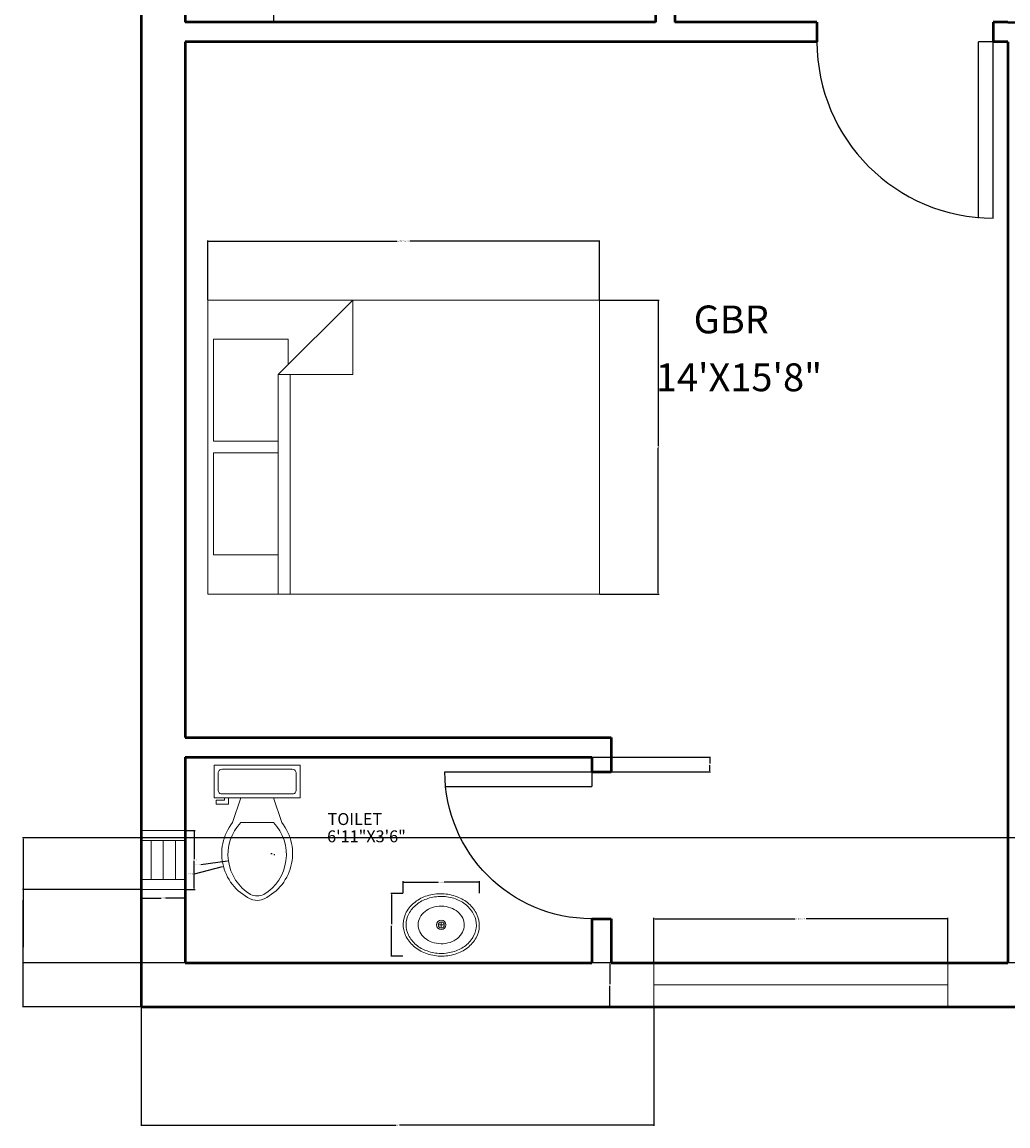
# Model space of a CAD drawing. Units: inches. Extents: x 66 to 499, y 601 to 1111.
# Tile 1 of 4: x 66 to 268, y 601 to 826. Entities that reach past the tile are written whole.
import ezdxf

# ---------------------------------------------------------------- set-up
doc = ezdxf.new("R2010")
doc.units = ezdxf.units.IN
for name, color, linetype, lineweight in [('A-ANNO-DIMS', 2, 'Continuous', 18), ('A-AREA-IDEN', 7, 'Continuous', 18), ('A-DOOR', 3, 'Continuous', 25), ('A-FLOR-CASE', 9, 'Continuous', 25), ('A-FLOR-FIXT', 9, 'Continuous', 18), ('A-FURN', 8, 'Continuous', 18), ('A-GLAZ', 4, 'Continuous', 18), ('A-WALL', 7, 'Continuous', 50)]:
    doc.layers.add(name, color=color, linetype=linetype, lineweight=lineweight)
doc.styles.get("Standard").update_dxf_attribs({"font": 'arial.ttf'})
doc.dimstyles.get("Standard").update_dxf_attribs({"dimtxt": 0.18, "dimasz": 0.18, "dimexe": 0.18, "dimexo": 0.0625, "dimgap": 0.09, "dimtad": 0, "dimtih": 1, "dimtoh": 1, "dimdec": 4, "dimzin": 0, "dimdsep": 46, "dimtxsty": 'Standard', "dimcen": 0.09, "dimadec": 0, "dimazin": 0, "dimtfac": 1, "dimtdec": 4, "dimtofl": 0, "dimtmove": 0, "dimatfit": 3, "dimfxl": 1, "dimtolj": 1, "dimtzin": 0, "dimarcsym": 0})

# ---------------------------------------------------------------- blocks, each defined once
blk = doc.blocks.new('Toilet - top')
for p, q in [((9.5, -6), (9.5, -2)), ((-8, -8.5), (-8, -8)), ((-7, -8), (-7, -9.5)), ((-4, -8), (-6, -14)), ((4, -8), (6, -14)), ((-10, -8.5), (-8, -8.5)), ((-10, -9.5), (-10, -8.5)), ((-7, -9.5), (-10, -9.5)), ((4, -14), (-4, -14))]:
    blk.add_line(p, q)
blk.add_lwpolyline([(10.5, -8), (10.5, 0), (-10.5, 0), (-10.5, -8)], close=True)
for points in [[(-9.5, -2), (-9.5, -6)], [(8.5, -1), (-8.5, -1)], [(-8.5, -7), (8.5, -7)]]:
    blk.add_lwpolyline(points)
for centre, radius, start, end in [((-8.62, -1.88), 0.884, 81.8699, 188.1301), ((8.62, -1.88), 0.884, 351.8699, 98.1301), ((-8.62, -6.12), 0.884, 171.8699, 278.1301), ((8.62, -6.12), 0.884, 261.8699, 8.1301), ((3.52, -21.58), 12.17, 141.4691, 247.9714), ((4.2, -21.82), 11.33, 136.3677, 238.9468), ((-3.52, -21.58), 12.17, 292.0284, 38.5307), ((-4.2, -21.82), 11.33, 301.053, 43.6321), ((0, -27.88), 4, 245.7318, 294.2682), ((0, -29), 4, 254.8605, 285.1395)]:
    blk.add_arc(centre, radius, start, end)
blk = doc.blocks.new('Sink - Oval top')
for p, q in [((-1, 0), (1, 0)), ((0, 1), (0, -1))]:
    blk.add_line(p, q)
for points in [[(-12.23, 0.39, 0.117634), (-11.46, -3.36, 0.104469), (-8.88, -6.8, 0.090016), (-5.08, -9.07, 0.08192), (-0.32, -10.02, 0.08192), (4.49, -9.38, 0.090016), (8.42, -7.36, 0.104469), (11.22, -4.09, 0.117634), (12.23, -0.39, 0.117634), (11.46, 3.36, 0.104469), (8.88, 6.8, 0.090016), (5.08, 9.07, 0.08192), (0.32, 10.02, 0.08192), (-4.49, 9.38, 0.090016), (-8.42, 7.36, 0.104469), (-11.22, 4.09, 0.117634)], [(-11.29, 0.16, 0.118622), (-10.52, -3.25, 0.104678), (-8.07, -6.36, 0.089562), (-4.54, -8.37, 0.081185), (-0.13, -9.15, 0.081185), (4.3, -8.49, 0.089562), (7.89, -6.58, 0.104678), (10.42, -3.55, 0.118622), (11.29, -0.16, 0.118622), (10.52, 3.25, 0.104678), (8.07, 6.36, 0.089562), (4.54, 8.37, 0.081185), (0.13, 9.15, 0.081185), (-4.3, 8.49, 0.089562), (-7.89, 6.58, 0.104678), (-10.42, 3.55, 0.118622)], [(-7.42, 0.08, 0.118283), (-6.91, -2.17, 0.104607), (-5.29, -4.21, 0.089718), (-2.97, -5.53, 0.081436), (-0.07, -6.04, 0.081436), (2.84, -5.59, 0.089718), (5.2, -4.33, 0.104607), (6.86, -2.32, 0.118283), (7.42, -0.08, 0.118283), (6.91, 2.17, 0.104607), (5.29, 4.21, 0.089718), (2.97, 5.53, 0.081436), (0.07, 6.04, 0.081436), (-2.84, 5.59, 0.089718), (-5.2, 4.33, 0.104607), (-6.86, 2.32, 0.118283)]]:
    blk.add_lwpolyline(points, format="xyb", close=True)
for radius in [1.5, 1]:
    blk.add_circle((0, 0), radius)
blk = doc.blocks.new('Bed - Queen')
for p, q in [((0, -80.00003), (0, 0)), ((0, 0), (59.99999, 0)), ((59.99999, 0), (59.99999, -80.00003)), ((7.99999, -1.2), (28.79998, -1.2)), ((7.99999, -14.4), (7.99999, -1.2)), ((28.79998, -1.2), (28.79998, -14.4)), ((31.19999, -1.2), (51.99999, -1.2)), ((31.19999, -14.4), (31.19999, -1.2)), ((51.99999, -1.2), (51.99999, -16.4)), ((0, -14.4), (44.8, -14.4)), ((59.99999, -29.6), (44.8, -14.4)), ((44.8, -14.4), (44.8, -29.6)), ((44.8, -16.8), (0, -16.8)), ((51.99999, -16.4), (46.79936, -16.4)), ((44.8, -29.6), (59.99999, -29.6)), ((59.99999, -80.00003), (0, -80.00003))]:
    blk.add_line(p, q)
blk = doc.blocks.new('DOOR-SWING-36IN')
for p, q in [((0, 36), (0, 0)), ((3, 36), (3, 0)), ((0, 0), (3, 0))]:
    blk.add_line(p, q)
blk.add_arc((0, 0), 36, 0, 90)
blk = doc.blocks.new('DOOR-SWING-30IN')
for p, q in [((0, 30), (0, 0)), ((3, 30), (3, 0)), ((0, 0), (3, 0.01))]:
    blk.add_line(p, q)
blk.add_arc((0, 0), 30, 0.0977, 90)
blk = doc.blocks.new('WIN-60IN')
for p, q in [((60, 9), (0, 9)), ((0, 9), (0, 0)), ((60, 0), (60, 9)), ((0, 4.5), (60, 4.5)), ((0, 0), (60, 0))]:
    blk.add_line(p, q)
blk = doc.blocks.new('WIN-BATH-VENT-12IN')
for p, q in [((0, 12), (0, 0)), ((9, 12), (0, 12)), ((9, 0), (9, 12)), ((9, 10), (0, 10)), ((2, 10), (2, 2)), ((4.5, 10), (4.5, 2)), ((7, 2), (7, 10)), ((0, 2), (9, 2)), ((0, 0), (9, 0))]:
    blk.add_line(p, q)
blk = doc.blocks.new('*D14')
at = {"layer": 'A-ANNO-DIMS', "color": 0, "lineweight": -2, "transparency": 16777216}
for p, q in [((195.27, 634.07), (195.27, 643.18)), ((195.45, 643), (224.15, 643)), ((255.09, 643), (226.39, 643)), ((255.27, 634.07), (255.27, 643.18))]:
    blk.add_line(p, q, dxfattribs=at)
at = {"layer": 'A-ANNO-DIMS', "color": 0, "transparency": 16777216}
for points in [[(195.45, 643.03), (195.45, 642.97), (195.27, 643)], [(255.09, 643.03), (255.09, 642.97), (255.27, 643)]]:
    blk.add_solid(points, dxfattribs=at)
at = {"layer": 'Defpoints', "color": 0, "transparency": 16777216}
for p in [(255.27, 643), (195.27, 634), (255.27, 634)]:
    blk.add_point(p, dxfattribs=at)
at = {"layer": 'A-ANNO-DIMS', "color": 0, "transparency": 16777216, "insert": (225.27, 643), "char_height": 0.18, "attachment_point": 5}
blk.add_mtext('\\A1;WINDOW 60 TYP.', dxfattribs=at)
blk = doc.blocks.new('*D15')
at = {"layer": 'A-ANNO-DIMS', "color": 0, "lineweight": -2, "transparency": 16777216}
for p, q in [((195.21, 634), (186.09, 634)), ((186.27, 633.82), (186.27, 629.69)), ((186.27, 625.18), (186.27, 629.32)), ((195.21, 625), (186.09, 625))]:
    blk.add_line(p, q, dxfattribs=at)
at = {"layer": 'A-ANNO-DIMS', "color": 0, "transparency": 16777216}
for points in [[(186.24, 633.82), (186.3, 633.82), (186.27, 634)], [(186.24, 625.18), (186.3, 625.18), (186.27, 625)]]:
    blk.add_solid(points, dxfattribs=at)
at = {"layer": 'Defpoints', "color": 0, "transparency": 16777216}
for p in [(186.27, 634), (195.27, 634), (195.27, 625)]:
    blk.add_point(p, dxfattribs=at)
at = {"layer": 'A-ANNO-DIMS', "color": 0, "transparency": 16777216, "insert": (186.27, 629.5), "char_height": 0.18, "attachment_point": 5}
blk.add_mtext('\\A1;9 TYP.', dxfattribs=at)
blk = doc.blocks.new('*D16')
at = {"layer": 'A-ANNO-DIMS', "color": 0, "lineweight": -2, "transparency": 16777216}
for p, q in [((104.16, 769.34), (104.16, 781.45)), ((104.34, 781.27), (142.86, 781.27)), ((183.98, 781.27), (145.46, 781.27)), ((184.16, 769.34), (184.16, 781.45))]:
    blk.add_line(p, q, dxfattribs=at)
at = {"layer": 'A-ANNO-DIMS', "color": 0, "transparency": 16777216}
for points in [[(104.34, 781.3), (104.34, 781.24), (104.16, 781.27)], [(183.98, 781.3), (183.98, 781.24), (184.16, 781.27)]]:
    blk.add_solid(points, dxfattribs=at)
at = {"layer": 'Defpoints', "color": 0, "transparency": 16777216}
for p in [(104.16, 781.27), (104.16, 769.27), (184.16, 769.27)]:
    blk.add_point(p, dxfattribs=at)
at = {"layer": 'A-ANNO-DIMS', "color": 0, "transparency": 16777216, "insert": (144.16, 781.27), "char_height": 0.18, "attachment_point": 5}
blk.add_mtext('\\A1;QUEEN BED 80 TYP.', dxfattribs=at)
blk = doc.blocks.new('*D17')
at = {"layer": 'A-ANNO-DIMS', "color": 0, "lineweight": -2, "transparency": 16777216}
for p, q in [((184.22, 769.27), (196.34, 769.27)), ((196.16, 769.09), (196.16, 739.46)), ((196.16, 709.45), (196.16, 739.09)), ((184.22, 709.27), (196.34, 709.27))]:
    blk.add_line(p, q, dxfattribs=at)
at = {"layer": 'A-ANNO-DIMS', "color": 0, "transparency": 16777216}
for points in [[(196.13, 769.09), (196.19, 769.09), (196.16, 769.27)], [(196.13, 709.45), (196.19, 709.45), (196.16, 709.27)]]:
    blk.add_solid(points, dxfattribs=at)
at = {"layer": 'Defpoints', "color": 0, "transparency": 16777216}
for p in [(184.16, 769.27), (196.16, 769.27), (184.16, 709.27)]:
    blk.add_point(p, dxfattribs=at)
at = {"layer": 'A-ANNO-DIMS', "color": 0, "transparency": 16777216, "insert": (196.16, 739.27), "char_height": 0.18, "attachment_point": 5}
blk.add_mtext('\\A1;60 TYP.', dxfattribs=at)
blk = doc.blocks.new('*D22')
at = {"layer": 'A-ANNO-DIMS', "color": 0, "lineweight": -2, "transparency": 16777216}
for p, q in [((144.04, 648.2), (144.04, 650.66)), ((144.22, 650.48), (151.21, 650.48)), ((159.46, 650.48), (152.47, 650.48)), ((159.64, 648.2), (159.64, 650.66))]:
    blk.add_line(p, q, dxfattribs=at)
at = {"layer": 'A-ANNO-DIMS', "color": 0, "transparency": 16777216}
for points in [[(144.22, 650.51), (144.22, 650.45), (144.04, 650.48)], [(159.46, 650.51), (159.46, 650.45), (159.64, 650.48)]]:
    blk.add_solid(points, dxfattribs=at)
at = {"layer": 'Defpoints', "color": 0, "transparency": 16777216}
for p in [(159.64, 650.48), (144.04, 648.14), (159.64, 648.14)]:
    blk.add_point(p, dxfattribs=at)
at = {"layer": 'A-ANNO-DIMS', "color": 0, "transparency": 16777216, "insert": (151.84, 650.48), "char_height": 0.18, "attachment_point": 5}
blk.add_mtext('\\A1;BASIN 16', dxfattribs=at)
blk = doc.blocks.new('*D23')
at = {"layer": 'A-ANNO-DIMS', "color": 0, "lineweight": -2, "transparency": 16777216}
for p, q in [((143.98, 648.14), (141.52, 648.14)), ((141.7, 647.96), (141.7, 641.93)), ((141.7, 635.52), (141.7, 641.56)), ((143.98, 635.34), (141.52, 635.34))]:
    blk.add_line(p, q, dxfattribs=at)
at = {"layer": 'A-ANNO-DIMS', "color": 0, "transparency": 16777216}
for points in [[(141.67, 647.96), (141.73, 647.96), (141.7, 648.14)], [(141.67, 635.52), (141.73, 635.52), (141.7, 635.34)]]:
    blk.add_solid(points, dxfattribs=at)
at = {"layer": 'Defpoints', "color": 0, "transparency": 16777216}
for p in [(141.7, 648.14), (144.04, 648.14), (144.04, 635.34)]:
    blk.add_point(p, dxfattribs=at)
at = {"layer": 'A-ANNO-DIMS', "color": 0, "transparency": 16777216, "insert": (141.7, 641.74), "char_height": 0.18, "attachment_point": 5}
blk.add_mtext('\\A1;13', dxfattribs=at)
blk = doc.blocks.new('*D30')
at = {"layer": 'A-ANNO-DIMS', "color": 0, "lineweight": -2, "transparency": 16777216}
for p, q in [((99.64, 661), (101.56, 661)), ((101.38, 660.82), (101.38, 655.18)), ((101.38, 649.18), (101.38, 654.82)), ((99.64, 649), (101.56, 649))]:
    blk.add_line(p, q, dxfattribs=at)
at = {"layer": 'A-ANNO-DIMS', "color": 0, "transparency": 16777216}
for points in [[(101.35, 660.82), (101.41, 660.82), (101.38, 661)], [(101.35, 649.18), (101.41, 649.18), (101.38, 649)]]:
    blk.add_solid(points, dxfattribs=at)
at = {"layer": 'Defpoints', "color": 0, "transparency": 16777216}
for p in [(99.58, 661), (101.38, 661), (99.58, 649)]:
    blk.add_point(p, dxfattribs=at)
at = {"layer": 'A-ANNO-DIMS', "color": 0, "transparency": 16777216, "insert": (101.38, 655), "char_height": 0.18, "attachment_point": 5}
blk.add_mtext('\\A1;VENT 12 TYP.', dxfattribs=at)
blk = doc.blocks.new('*D31')
at = {"layer": 'A-ANNO-DIMS', "color": 0, "lineweight": -2, "transparency": 16777216}
for p, q in [((90.58, 648.94), (90.58, 647.02)), ((99.58, 648.94), (99.58, 647.02)), ((90.76, 647.2), (94.62, 647.2)), ((99.4, 647.2), (95.53, 647.2))]:
    blk.add_line(p, q, dxfattribs=at)
at = {"layer": 'A-ANNO-DIMS', "color": 0, "transparency": 16777216}
for points in [[(90.76, 647.23), (90.76, 647.17), (90.58, 647.2)], [(99.4, 647.23), (99.4, 647.17), (99.58, 647.2)]]:
    blk.add_solid(points, dxfattribs=at)
at = {"layer": 'Defpoints', "color": 0, "transparency": 16777216}
for p in [(90.58, 649), (99.58, 649), (99.58, 647.2)]:
    blk.add_point(p, dxfattribs=at)
at = {"layer": 'A-ANNO-DIMS', "color": 0, "transparency": 16777216, "insert": (95.08, 647.2), "char_height": 0.18, "attachment_point": 5}
blk.add_mtext('\\A1;9 TYP.', dxfattribs=at)
blk = doc.blocks.new('*D47')
at = {"layer": 'A-ANNO-DIMS', "color": 0, "lineweight": -2, "transparency": 16777216}
for p, q in [((90.58, 624.94), (90.58, 600.72)), ((195.27, 624.94), (195.27, 600.72)), ((90.76, 600.9), (142.54, 600.9)), ((195.09, 600.9), (143.31, 600.9))]:
    blk.add_line(p, q, dxfattribs=at)
at = {"layer": 'A-ANNO-DIMS', "color": 0, "transparency": 16777216}
for points in [[(90.76, 600.93), (90.76, 600.87), (90.58, 600.9)], [(195.09, 600.93), (195.09, 600.87), (195.27, 600.9)]]:
    blk.add_solid(points, dxfattribs=at)
at = {"layer": 'Defpoints', "color": 0, "transparency": 16777216}
for p in [(90.58, 625), (195.27, 625), (195.27, 600.9)]:
    blk.add_point(p, dxfattribs=at)
at = {"layer": 'A-ANNO-DIMS', "color": 0, "transparency": 16777216, "insert": (142.92, 600.9), "char_height": 0.18, "attachment_point": 5}
blk.add_mtext('\\A1;104.7', dxfattribs=at)
blk = doc.blocks.new('*D49')
at = {"layer": 'A-ANNO-DIMS', "color": 0, "lineweight": -2, "transparency": 16777216}
for p, q in [((90.51, 649), (66.3, 649)), ((66.48, 648.82), (66.48, 637.18)), ((66.48, 625.18), (66.48, 636.82)), ((90.51, 625), (66.3, 625))]:
    blk.add_line(p, q, dxfattribs=at)
at = {"layer": 'A-ANNO-DIMS', "color": 0, "transparency": 16777216}
for points in [[(66.45, 648.82), (66.51, 648.82), (66.48, 649)], [(66.45, 625.18), (66.51, 625.18), (66.48, 625)]]:
    blk.add_solid(points, dxfattribs=at)
at = {"layer": 'Defpoints', "color": 0, "transparency": 16777216}
for p in [(66.48, 649), (90.58, 649), (90.58, 625)]:
    blk.add_point(p, dxfattribs=at)
at = {"layer": 'A-ANNO-DIMS', "color": 0, "transparency": 16777216, "insert": (66.48, 637), "char_height": 0.18, "attachment_point": 5}
blk.add_mtext('\\A1;24', dxfattribs=at)
blk = doc.blocks.new('*D54')
at = {"layer": 'A-ANNO-DIMS', "color": 0, "lineweight": -2, "transparency": 16777216}
for p, q in [((358.51, 659.5), (66.3, 659.5)), ((66.48, 659.32), (66.48, 646.94)), ((66.48, 634.18), (66.48, 646.57)), ((358.51, 634), (66.3, 634))]:
    blk.add_line(p, q, dxfattribs=at)
at = {"layer": 'A-ANNO-DIMS', "color": 0, "transparency": 16777216}
for points in [[(66.45, 659.32), (66.51, 659.32), (66.48, 659.5)], [(66.45, 634.18), (66.51, 634.18), (66.48, 634)]]:
    blk.add_solid(points, dxfattribs=at)
at = {"layer": 'Defpoints', "color": 0, "transparency": 16777216}
for p in [(66.48, 659.5), (358.58, 659.5), (358.58, 634)]:
    blk.add_point(p, dxfattribs=at)
at = {"layer": 'A-ANNO-DIMS', "color": 0, "transparency": 16777216, "insert": (66.48, 646.75), "char_height": 0.18, "attachment_point": 5}
blk.add_mtext('\\A1;25.5', dxfattribs=at)
blk = doc.blocks.new('*D67')
at = {"layer": 'A-ANNO-DIMS', "color": 0, "lineweight": -2, "transparency": 16777216}
for p, q in [((182.64, 676), (206.86, 676)), ((206.68, 675.82), (206.68, 674.69)), ((206.68, 673.18), (206.68, 674.32)), ((182.64, 673), (206.86, 673))]:
    blk.add_line(p, q, dxfattribs=at)
at = {"layer": 'A-ANNO-DIMS', "color": 0, "transparency": 16777216}
for points in [[(206.65, 675.82), (206.71, 675.82), (206.68, 676)], [(206.65, 673.18), (206.71, 673.18), (206.68, 673)]]:
    blk.add_solid(points, dxfattribs=at)
at = {"layer": 'Defpoints', "color": 0, "transparency": 16777216}
for p in [(182.58, 676), (182.58, 673), (206.68, 673)]:
    blk.add_point(p, dxfattribs=at)
at = {"layer": 'A-ANNO-DIMS', "color": 0, "transparency": 16777216, "insert": (206.68, 674.5), "char_height": 0.18, "attachment_point": 5}
blk.add_mtext('\\A1;3', dxfattribs=at)
blk = doc.blocks.new('*D70')
at = {"layer": 'A-ANNO-DIMS', "color": 0, "lineweight": -2, "transparency": 16777216}
for p, q in [((117.11, 656.29), (117.29, 656.29)), ((117.2, 656.2), (117.2, 656.38)), ((101.45, 652.16), (107.18, 653.66))]:
    blk.add_line(p, q, dxfattribs=at)
at = {"layer": 'A-ANNO-DIMS', "color": 0, "transparency": 16777216}
blk.add_solid([(107.17, 653.69), (107.19, 653.63), (107.36, 653.71)], dxfattribs=at)
at = {"layer": 'Defpoints', "color": 0, "transparency": 16777216}
for p in [(117.2, 656.29), (107.36, 653.71)]:
    blk.add_point(p, dxfattribs=at)
at = {"layer": 'A-ANNO-DIMS', "color": 0, "transparency": 16777216, "insert": (100.7, 652.16), "char_height": 0.18, "attachment_point": 5}
blk.add_mtext('\\A1;4X R10.176', dxfattribs=at)
blk = doc.blocks.new('*D71')
at = {"layer": 'A-ANNO-DIMS', "color": 0, "lineweight": -2, "transparency": 16777216}
for p, q in [((117.68, 656.09), (117.86, 656.09)), ((117.77, 656), (117.77, 656.18)), ((102.74, 654.07), (108.2, 654.81))]:
    blk.add_line(p, q, dxfattribs=at)
at = {"layer": 'A-ANNO-DIMS', "color": 0, "transparency": 16777216}
blk.add_solid([(108.19, 654.84), (108.2, 654.78), (108.38, 654.83)], dxfattribs=at)
at = {"layer": 'Defpoints', "color": 0, "transparency": 16777216}
for p in [(117.77, 656.09), (108.38, 654.83)]:
    blk.add_point(p, dxfattribs=at)
at = {"layer": 'A-ANNO-DIMS', "color": 0, "transparency": 16777216, "insert": (102.07, 654.07), "char_height": 0.18, "attachment_point": 5}
blk.add_mtext('\\A1;4X R9.474', dxfattribs=at)

msp = doc.modelspace()

# ---------------------------------------------------------------- linework, layer by layer
at = {"layer": 'A-FLOR-CASE'}
msp.add_line((117.5757, 910.0042), (117.5757, 826.0042), dxfattribs=at)
at = {"layer": 'A-WALL'}
for p, q in [((99.5757, 928.0042), (99.5757, 826.0042)), ((195.5757, 895.0042), (195.5757, 826.0042)), ((199.5757, 895.0042), (199.5757, 826.0042)), ((195.5757, 826.0042), (99.5757, 826.0042)), ((228.5757, 826.0042), (199.5757, 826.0042)), ((228.5757, 826.0042), (228.5757, 822.0042)), ((267.5757, 826.0042), (264.5757, 826.0042)), ((264.5757, 826.0042), (264.5757, 822.0042)), ((267.5757, 826.0042), (273.5757, 825.9236)), ((228.5757, 822.0042), (99.5757, 822.0042)), ((99.5757, 822.0042), (99.5757, 680.0042)), ((267.5757, 822.0042), (264.5757, 822.0042)), ((267.5757, 822.0042), (267.5757, 634.0042)), ((99.5757, 680.0042), (186.5757, 680.0042)), ((186.5757, 680.0042), (186.5757, 673.0042)), ((99.5757, 676.0042), (182.5757, 676.0042)), ((99.5757, 676.0042), (99.5757, 634.0042)), ((182.5757, 676.0042), (182.5757, 673.0042)), ((182.5757, 673.0042), (186.5757, 673.0042)), ((182.5757, 643.0042), (186.5757, 643.0042)), ((182.5757, 643.0042), (182.5757, 634.0042)), ((186.5757, 643.0042), (186.5757, 634.0042)), ((99.5757, 634.0042), (182.5757, 634.0042)), ((186.5757, 634.0042), (267.5757, 634.0042))]:
    msp.add_line(p, q, dxfattribs=at)
msp.add_lwpolyline([(90.5757, 625.0042), (474.5757, 625.0042), (474.5757, 1087.0042), (90.5757, 1087.0042)], close=True, dxfattribs=at)

# ---------------------------------------------------------------- block references
at = {"layer": 'A-DOOR', "rotation": 180}
msp.add_blockref('DOOR-SWING-36IN', (264.5757, 822.0042), dxfattribs=at)
at = {"layer": 'A-DOOR', "extrusion": (0, 0, -1), "zscale": -1, "rotation": 270.0000000000051}
msp.add_blockref('DOOR-SWING-30IN', (-182.5757, 673.0042), dxfattribs=at)
at = {"layer": 'A-FLOR-FIXT'}
for name, p, xscale, yscale, zscale in [('Toilet - top', (114.2546, 674.3396), 0.8362564653676912, 0.8362564653676912, 0.8362564653676912), ('Sink - Oval top', (151.839, 641.7435), 0.6355214176072885, 0.6355214176072885, 0.6355214176072885)]:
    msp.add_blockref(name, p, dxfattribs=dict(at, xscale=xscale, yscale=yscale, zscale=zscale))
at = {"layer": 'A-FURN', "rotation": 90}
msp.add_blockref('Bed - Queen', (104.1603, 709.2738), dxfattribs=at)
at = {"layer": 'A-GLAZ'}
for name, p in [('WIN-BATH-VENT-12IN', (90.5757, 649.0042)), ('WIN-60IN', (195.2689, 625.0042))]:
    msp.add_blockref(name, p, dxfattribs=at)

# ---------------------------------------------------------------- texts
at = {"layer": 'A-AREA-IDEN', "attachment_point": 1}
for s, width, gutter_width, insert, char_height in [('GBR', 58.656418, 28.4105, (203.3877, 768.1581), 5.6821), ('14\'X15\'8"', 58.656418, 28.4105, (195.6801, 756.3498), 5.6821), ('TOILET', 25.071112, 12.1433, (128.6315, 664.567), 2.42866), ('6\'11"X3\'6"', 25.071112, 12.1433, (128.5398, 661.0403), 2.42866)]:
    msp.add_mtext_dynamic_manual_height_columns(s, width=width, gutter_width=gutter_width, heights=[0], dxfattribs=dict(at, insert=insert, char_height=char_height))

# ---------------------------------------------------------------- dimensions: what is measured, and where the dimension line sits
at = {"layer": 'A-ANNO-DIMS'}
for base, p1, p2, angle, text, picture, middle in [((104.1603, 781.2738), (184.1603, 769.2738), (104.1603, 769.2738), 180, 'QUEEN BED <> TYP.', '*D16', (144.1603, 781.2738)), ((196.1603, 769.2738), (184.1603, 709.2738), (184.1603, 769.2738), 90, '<> TYP.', '*D17', (196.1603, 739.2738)), ((101.3757, 661.0042), (99.5757, 649.0042), (99.5757, 661.0042), 90, 'VENT <> TYP.', '*D30', (101.3757, 655.0042)), ((186.2689, 634.0042), (195.2689, 625.0042), (195.2689, 634.0042), 90, '<> TYP.', '*D15', (186.2689, 629.5042))]:
    dim = msp.add_linear_dim(base=base, p1=p1, p2=p2, angle=angle, text=text, dimstyle='Standard', override={"dimdec": 0, "dimlfac": 1, "dimrnd": 0, "dimzin": 0, "dimdsep": 46, "dimlunit": 2}, dxfattribs=at)
    dim.commit()
    dim.dimension.update_dxf_attribs({"geometry": picture, "text_midpoint": middle})
for base, p1, p2, angle, override, picture, middle in [((206.6757, 673.0042), (182.5757, 676.0042), (182.5757, 673.0042), 270, {"dimdec": 0, "dimlfac": 1, "dimrnd": 0, "dimzin": 0, "dimdsep": 46, "dimlunit": 2}, '*D67', (206.6757, 674.5042)), ((66.4757, 659.5042), (358.5757, 634.0042), (358.5757, 659.5042), 90, {"dimdec": 1, "dimlfac": 1, "dimrnd": 0, "dimzin": 0, "dimdsep": 46, "dimlunit": 2}, '*D54', (66.4757, 646.7542)), ((66.4757, 649.0042), (90.5757, 625.0042), (90.5757, 649.0042), 90, {"dimdec": 0, "dimlfac": 1, "dimrnd": 0, "dimzin": 0, "dimdsep": 46, "dimlunit": 2}, '*D49', (66.4757, 637.0042)), ((141.6973, 648.1421), (144.0377, 635.3448), (144.0377, 648.1421), 90, {"dimdec": 0, "dimlfac": 1, "dimrnd": 0, "dimzin": 0, "dimdsep": 46, "dimlunit": 2}, '*D23', (141.6973, 641.7435))]:
    dim = msp.add_linear_dim(base=base, p1=p1, p2=p2, angle=angle, dimstyle='Standard', override=override, dxfattribs=at)
    dim.commit()
    dim.dimension.update_dxf_attribs({"geometry": picture, "text_midpoint": middle})
for center, mpoint, picture, middle in [((117.1979, 656.2928), (107.3554, 653.7071), '*D70', (101.45, 652.1557)), ((117.7669, 656.0947), (108.3773, 654.832), '*D71', (102.7435, 654.0745))]:
    dim = msp.add_radius_dim(center=center, mpoint=mpoint, text='4X <>', dimstyle='Standard', override={"dimdec": 3, "dimlfac": 1, "dimrnd": 0, "dimzin": 0, "dimdsep": 46, "dimlunit": 2}, dxfattribs=at)
    dim.commit()
    dim.dimension.update_dxf_attribs({"geometry": picture, "text_midpoint": middle, "dimtype": 164})
for base, p1, p2, text, picture, middle in [((99.5757, 647.2042), (90.5757, 649.0042), (99.5757, 649.0042), '<> TYP.', '*D31', (95.0757, 647.2042)), ((159.6403, 650.4825), (144.0377, 648.1421), (159.6403, 648.1421), 'BASIN <>', '*D22', (151.839, 650.4825)), ((255.2689, 643.0042), (195.2689, 634.0042), (255.2689, 634.0042), 'WINDOW <> TYP.', '*D14', (225.2689, 643.0042))]:
    dim = msp.add_linear_dim(base=base, p1=p1, p2=p2, text=text, dimstyle='Standard', override={"dimdec": 0, "dimlfac": 1, "dimrnd": 0, "dimzin": 0, "dimdsep": 46, "dimlunit": 2}, dxfattribs=at)
    dim.commit()
    dim.dimension.update_dxf_attribs({"geometry": picture, "text_midpoint": middle})
dim = msp.add_linear_dim(base=(195.2689, 600.9042), p1=(90.5757, 625.0042), p2=(195.2689, 625.0042), dimstyle='Standard', override={"dimdec": 1, "dimlfac": 1, "dimrnd": 0, "dimzin": 0, "dimdsep": 46, "dimlunit": 2}, dxfattribs=at)
dim.commit()
dim.dimension.update_dxf_attribs({"geometry": '*D47', "text_midpoint": (142.9223, 600.9042)})

doc.saveas('drawing.dxf')
